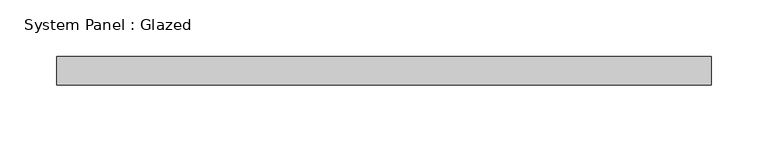
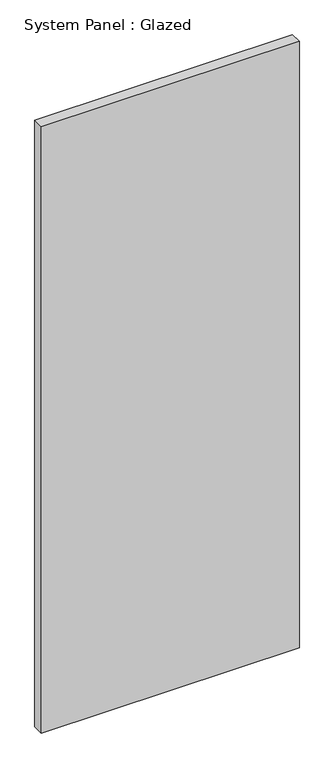
"""IFC4 building model written with IfcOpenShell, lengths in millimetres: plate geometry, System Panel : Glazed."""

from ifc_helpers import new_model, si_unit, origin, origin_with_axes, place, context, project, spatial, polyline, outline, extrude, source, transform, mapped, element, save


def system_panel_glazed_37901f3f(model_context):
    return source(origin(), model_context, "Body", "SweptSolid", [
        extrude(outline(polyline([(288.925, 19.05), (-288.925, 19.05), (-288.925, 44.45), (288.925, 44.45), (288.925, 19.05)])), origin_with_axes(), (0.0, 0.0, 1.0), 1435.1313909),
    ])


if __name__ == "__main__":
    model = new_model("IFC4")
    model_context = context("Model", 3, world=origin())
    ifc_project = project(units=[si_unit("LENGTHUNIT", "METRE", prefix="MILLI")], contexts=[model_context])
    site = spatial("IfcSite", under=ifc_project)
    building = spatial("IfcBuilding", under=site)
    placement = place(None, origin())
    system_panel_glazed_shape = system_panel_glazed_37901f3f(model_context)
    element("IfcPlate", 1, ObjectType="System Panel : Glazed", at=placement, inside=building, context=model_context, shape_type="MappedRepresentation", body=[
        mapped(system_panel_glazed_shape, transform((0.0, 0.0, 0.0), x_axis=(1.0, 0.0, 0.0), y_axis=(0.0, 1.0, 0.0), z_axis=(0.0, 0.0, 1.0))),
    ])
    save(model, "model.ifc")

# Revit data of these elements
# Type "System Panel : Glazed"
#   Construction Type Id = "GSP4R"
#   Analytic Construction = "1/8 in Pilkington single glazing"
#   Visual Light Transmittance = 0.9
#   Solar Heat Gain Coefficient = 0.86
#   Heat Transfer Coefficient (U) = 1.18115 BTU/(h·ft²·°F)
#   Define Thermal Properties by = 1
# Element 1 (IfcPlate, "System Panel : Glazed")
#   Materials on its faces: "Glass"
# Materials
#   "Glass": class "Glass", colour RGB 0 128 192, transparency 0.75, Description = "Soda Lime Glass", Cost = 0
